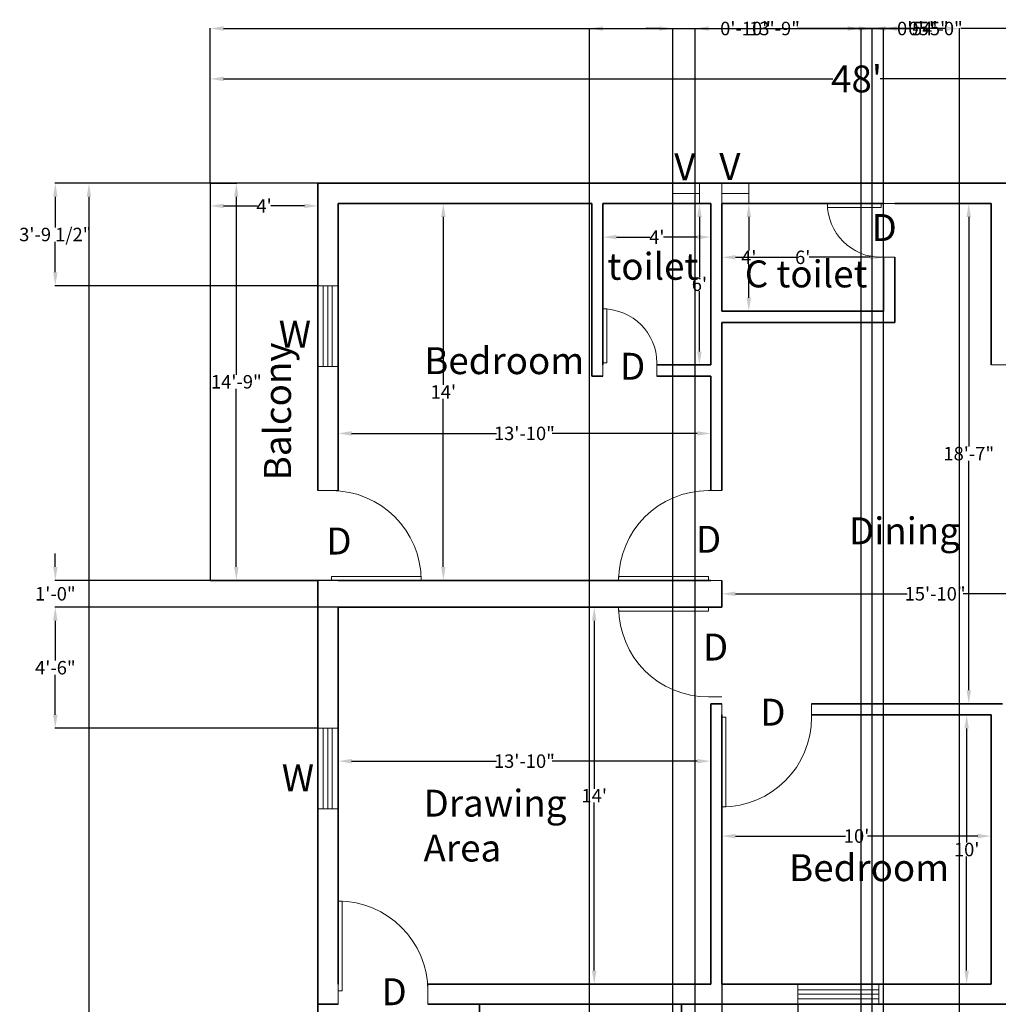
# Model space of a CAD drawing. Units: inches. Extents: x 1936 to 2761, y 1431 to 2889.
# Tile 5 of 6: x 1936 to 2372, y 2451 to 2889. Entities that reach past the tile are written whole.
import ezdxf

# ---------------------------------------------------------------- set-up
doc = ezdxf.new("R2010")
doc.units = ezdxf.units.IN
doc.header["$MEASUREMENT"] = 0
for name, color, linetype, lineweight in [('A-ANNO-DIMS', 172, 'Continuous', 13), ('A-ANNO-TEXT', 50, 'Continuous', 18), ('A-AREA-IDEN', 50, 'Continuous', 18), ('A-FLOR-EDGE', 4, 'Continuous', 25), ('A-FLOR-EVTR', 4, 'Continuous', 35), ('A-FLOR-FIXT', 8, 'Continuous', 18), ('A-GLAZ', 3, 'Continuous', 18), ('A-WALL', 4, 'Continuous', 35), ('doors', 10, 'Continuous', 18)]:
    doc.layers.add(name, color=color, linetype=linetype, lineweight=lineweight)
doc.styles.get("Standard").update_dxf_attribs({"font": 'arial.ttf'})
doc.dimstyles.get("Standard").update_dxf_attribs({"dimtxt": 6, "dimasz": 6, "dimexe": 0.18, "dimexo": 0.0625, "dimgap": 0.09, "dimtad": 0, "dimtih": 1, "dimtoh": 1, "dimdec": 0, "dimzin": 0, "dimdsep": 46, "dimlunit": 3, "dimtxsty": 'Standard', "dimcen": 0.09, "dimadec": 0, "dimazin": 0, "dimtfac": 1, "dimtdec": 0, "dimtofl": 0, "dimtmove": 0, "dimatfit": 3, "dimfxl": 1, "dimtolj": 1, "dimtzin": 0, "dimarcsym": 0})

# ---------------------------------------------------------------- blocks, each defined once
blk = doc.blocks.new('*U4')
for p, q in [((0, 0), (0, 6)), ((24, 0), (24, 6))]:
    blk.add_line(p, q)
blk.add_lwpolyline([(0, 0), (0, -24), (1.75, -24), (1.75, 0)], close=True)
blk.add_arc((0, 0), 24, 270, 0)
blk = doc.blocks.new('*U3')
for p, q in [((0, 0), (0, -6)), ((24, 0), (24, -6))]:
    blk.add_line(p, q)
blk.add_lwpolyline([(0, 0), (0, 24), (1.75, 24), (1.75, 0)], close=True)
blk.add_arc((0, 0), 24, 0, 90)
blk = doc.blocks.new('*U5')
for p, q in [((0, 0), (0, -6)), ((40, 0), (40, -6))]:
    blk.add_line(p, q)
blk.add_lwpolyline([(0, 0), (0, 40), (1.75, 40), (1.75, 0)], close=True)
blk.add_arc((0, 0), 40, 0, 90)
blk = doc.blocks.new('*U2')
for p, q in [((0, 0), (0, 6)), ((40, 0), (40, 6))]:
    blk.add_line(p, q)
blk.add_lwpolyline([(0, 0), (0, -40), (1.75, -40), (1.75, 0)], close=True)
blk.add_arc((0, 0), 40, 270, 360)
blk = doc.blocks.new('*U6')
for p, q in [((0, 0), (0, -6)), ((40, 0), (40, -6))]:
    blk.add_line(p, q)
blk.add_lwpolyline([(0, 0), (0, 40), (1.75, 40), (1.75, 0)], close=True)
blk.add_arc((0, 0), 40, 0, 90)
blk = doc.blocks.new('*U7')
for p, q in [((0, 0), (0, 6)), ((40, 0), (40, 6))]:
    blk.add_line(p, q)
blk.add_lwpolyline([(0, 0), (0, -40), (1.75, -40), (1.75, 0)], close=True)
blk.add_arc((0, 0), 40, 270, 0)
blk = doc.blocks.new('*D8')
at = {"layer": 'A-ANNO-DIMS', "color": 0, "lineweight": -2, "transparency": 16777216}
for p, q in [((2078.01, 2697.85), (2078.01, 2705.23)), ((2084.01, 2705.05), (2148.56, 2705.05)), ((2238.01, 2705.05), (2173.45, 2705.05)), ((2244.01, 2697.85), (2244.01, 2705.23))]:
    blk.add_line(p, q, dxfattribs=at)
at = {"layer": 'A-ANNO-DIMS', "color": 0, "transparency": 16777216}
for points in [[(2084.01, 2706.05), (2084.01, 2704.05), (2078.01, 2705.05)], [(2238.01, 2706.05), (2238.01, 2704.05), (2244.01, 2705.05)]]:
    blk.add_solid(points, dxfattribs=at)
at = {"layer": 'Defpoints', "color": 0, "transparency": 16777216}
for p in [(2244.01, 2705.05), (2078.01, 2697.79), (2244.01, 2697.79)]:
    blk.add_point(p, dxfattribs=at)
at = {"layer": 'A-ANNO-DIMS', "color": 0, "transparency": 16777216, "insert": (2161.01, 2705.05), "char_height": 6, "attachment_point": 5}
blk.add_mtext('\\A1;13\'-10"', dxfattribs=at)
blk = doc.blocks.new('*D9')
at = {"layer": 'A-ANNO-DIMS', "color": 0, "lineweight": -2, "transparency": 16777216}
for p, q in [((2124.95, 2807.55), (2125.07, 2807.55)), ((2124.89, 2801.55), (2124.89, 2726.65)), ((2124.89, 2645.55), (2124.89, 2720.45)), ((2124.95, 2639.55), (2125.07, 2639.55))]:
    blk.add_line(p, q, dxfattribs=at)
at = {"layer": 'A-ANNO-DIMS', "color": 0, "transparency": 16777216}
for points in [[(2123.89, 2801.55), (2125.89, 2801.55), (2124.89, 2807.55)], [(2123.89, 2645.55), (2125.89, 2645.55), (2124.89, 2639.55)]]:
    blk.add_solid(points, dxfattribs=at)
at = {"layer": 'Defpoints', "color": 0, "transparency": 16777216}
for p in [(2124.89, 2807.55), (2124.89, 2639.55), (2124.89, 2639.55)]:
    blk.add_point(p, dxfattribs=at)
at = {"layer": 'A-ANNO-DIMS', "color": 0, "transparency": 16777216, "insert": (2124.89, 2723.55), "char_height": 6, "attachment_point": 5}
blk.add_mtext("\\A1;14'", dxfattribs=at)
blk = doc.blocks.new('*D10')
at = {"layer": 'A-ANNO-DIMS', "color": 0, "lineweight": -2, "transparency": 16777216}
for p, q in [((2249.01, 2633.61), (2249.01, 2633.73)), ((2439.01, 2633.61), (2439.01, 2633.73)), ((2255.01, 2633.55), (2331.56, 2633.55)), ((2433.01, 2633.55), (2356.45, 2633.55))]:
    blk.add_line(p, q, dxfattribs=at)
at = {"layer": 'A-ANNO-DIMS', "color": 0, "transparency": 16777216}
for points in [[(2255.01, 2634.55), (2255.01, 2632.55), (2249.01, 2633.55)], [(2433.01, 2634.55), (2433.01, 2632.55), (2439.01, 2633.55)]]:
    blk.add_solid(points, dxfattribs=at)
at = {"layer": 'Defpoints', "color": 0, "transparency": 16777216}
for p in [(2249.01, 2633.55), (2439.01, 2633.55), (2439.01, 2633.55)]:
    blk.add_point(p, dxfattribs=at)
at = {"layer": 'A-ANNO-DIMS', "color": 0, "transparency": 16777216, "insert": (2344.01, 2633.55), "char_height": 6, "attachment_point": 5}
blk.add_mtext('\\A1;15\'-10"', dxfattribs=at)
blk = doc.blocks.new('*D11')
at = {"layer": 'A-ANNO-DIMS', "color": 0, "lineweight": -2, "transparency": 16777216}
for p, q in [((2347.57, 2807.55), (2359.19, 2807.55)), ((2359.01, 2801.55), (2359.01, 2699.2)), ((2359.01, 2590.55), (2359.01, 2692.9)), ((2347.57, 2584.55), (2359.19, 2584.55))]:
    blk.add_line(p, q, dxfattribs=at)
at = {"layer": 'A-ANNO-DIMS', "color": 0, "transparency": 16777216}
for points in [[(2358.01, 2801.55), (2360.01, 2801.55), (2359.01, 2807.55)], [(2358.01, 2590.55), (2360.01, 2590.55), (2359.01, 2584.55)]]:
    blk.add_solid(points, dxfattribs=at)
at = {"layer": 'Defpoints', "color": 0, "transparency": 16777216}
for p in [(2347.51, 2807.55), (2347.51, 2584.55), (2359.01, 2584.55)]:
    blk.add_point(p, dxfattribs=at)
at = {"layer": 'A-ANNO-DIMS', "color": 0, "transparency": 16777216, "insert": (2359.01, 2696.05), "char_height": 6, "attachment_point": 5}
blk.add_mtext('\\A1;18\'-7"', dxfattribs=at)
blk = doc.blocks.new('*D16')
at = {"layer": 'A-ANNO-DIMS', "color": 0, "lineweight": -2, "transparency": 16777216}
for p, q in [((2249.01, 2783.61), (2249.01, 2783.73)), ((2255.01, 2783.55), (2282.14, 2783.55)), ((2315.01, 2783.55), (2287.87, 2783.55)), ((2321.01, 2783.49), (2321.01, 2783.37))]:
    blk.add_line(p, q, dxfattribs=at)
at = {"layer": 'A-ANNO-DIMS', "color": 0, "transparency": 16777216}
for points in [[(2255.01, 2784.55), (2255.01, 2782.55), (2249.01, 2783.55)], [(2315.01, 2784.55), (2315.01, 2782.55), (2321.01, 2783.55)]]:
    blk.add_solid(points, dxfattribs=at)
at = {"layer": 'Defpoints', "color": 0, "transparency": 16777216}
for p in [(2249.01, 2783.55), (2321.01, 2783.55), (2321.01, 2783.55)]:
    blk.add_point(p, dxfattribs=at)
at = {"layer": 'A-ANNO-DIMS', "color": 0, "transparency": 16777216, "insert": (2285.01, 2783.55), "char_height": 6, "attachment_point": 5}
blk.add_mtext("\\A1;6'", dxfattribs=at)
blk = doc.blocks.new('*D17')
at = {"layer": 'A-ANNO-DIMS', "color": 0, "lineweight": -2, "transparency": 16777216}
for p, q in [((2261.07, 2807.55), (2261.19, 2807.55)), ((2261.01, 2801.55), (2261.01, 2786.64)), ((2261.01, 2765.55), (2261.01, 2780.46)), ((2261.07, 2759.55), (2261.19, 2759.55))]:
    blk.add_line(p, q, dxfattribs=at)
at = {"layer": 'A-ANNO-DIMS', "color": 0, "transparency": 16777216}
for points in [[(2260.01, 2801.55), (2262.01, 2801.55), (2261.01, 2807.55)], [(2260.01, 2765.55), (2262.01, 2765.55), (2261.01, 2759.55)]]:
    blk.add_solid(points, dxfattribs=at)
at = {"layer": 'Defpoints', "color": 0, "transparency": 16777216}
for p in [(2261.01, 2807.55), (2261.01, 2759.55), (2261.01, 2759.55)]:
    blk.add_point(p, dxfattribs=at)
at = {"layer": 'A-ANNO-DIMS', "color": 0, "transparency": 16777216, "insert": (2261.01, 2783.55), "char_height": 6, "attachment_point": 5}
blk.add_mtext("\\A1;4'", dxfattribs=at)
blk = doc.blocks.new('*D18')
at = {"layer": 'A-ANNO-DIMS', "color": 0, "lineweight": -2, "transparency": 16777216}
for p, q in [((2234.79, 2807.55), (2239.17, 2807.55)), ((2238.99, 2801.55), (2238.99, 2774.7)), ((2238.99, 2741.55), (2238.99, 2768.4)), ((2234.79, 2735.55), (2239.17, 2735.55))]:
    blk.add_line(p, q, dxfattribs=at)
at = {"layer": 'A-ANNO-DIMS', "color": 0, "transparency": 16777216}
for points in [[(2237.99, 2801.55), (2239.99, 2801.55), (2238.99, 2807.55)], [(2237.99, 2741.55), (2239.99, 2741.55), (2238.99, 2735.55)]]:
    blk.add_solid(points, dxfattribs=at)
at = {"layer": 'Defpoints', "color": 0, "transparency": 16777216}
for p in [(2234.73, 2807.55), (2234.73, 2735.55), (2238.99, 2735.55)]:
    blk.add_point(p, dxfattribs=at)
at = {"layer": 'A-ANNO-DIMS', "color": 0, "transparency": 16777216, "insert": (2238.99, 2771.55), "char_height": 6, "attachment_point": 5}
blk.add_mtext("\\A1;6'", dxfattribs=at)
blk = doc.blocks.new('*D19')
at = {"layer": 'A-ANNO-DIMS', "color": 0, "lineweight": -2, "transparency": 16777216}
for p, q in [((2196.01, 2792.63), (2196.01, 2792.74)), ((2202.01, 2792.56), (2217.03, 2792.56)), ((2238.01, 2792.56), (2222.98, 2792.56)), ((2244.01, 2792.63), (2244.01, 2792.74))]:
    blk.add_line(p, q, dxfattribs=at)
at = {"layer": 'A-ANNO-DIMS', "color": 0, "transparency": 16777216}
for points in [[(2202.01, 2793.56), (2202.01, 2791.56), (2196.01, 2792.56)], [(2238.01, 2793.56), (2238.01, 2791.56), (2244.01, 2792.56)]]:
    blk.add_solid(points, dxfattribs=at)
at = {"layer": 'Defpoints', "color": 0, "transparency": 16777216}
for p in [(2196.01, 2792.56), (2196.01, 2792.56), (2244.01, 2792.56)]:
    blk.add_point(p, dxfattribs=at)
at = {"layer": 'A-ANNO-DIMS', "color": 0, "transparency": 16777216, "insert": (2220.01, 2792.56), "char_height": 6, "attachment_point": 5}
blk.add_mtext("\\A1;4'", dxfattribs=at)
blk = doc.blocks.new('*D20')
at = {"layer": 'A-ANNO-DIMS', "color": 0, "lineweight": -2, "transparency": 16777216}
for p, q in [((2078.01, 2559.01), (2078.01, 2559.13)), ((2244.01, 2559.01), (2244.01, 2559.13)), ((2084.01, 2558.95), (2148.56, 2558.95)), ((2238.01, 2558.95), (2173.45, 2558.95))]:
    blk.add_line(p, q, dxfattribs=at)
at = {"layer": 'A-ANNO-DIMS', "color": 0, "transparency": 16777216}
for points in [[(2084.01, 2559.95), (2084.01, 2557.95), (2078.01, 2558.95)], [(2238.01, 2559.95), (2238.01, 2557.95), (2244.01, 2558.95)]]:
    blk.add_solid(points, dxfattribs=at)
at = {"layer": 'Defpoints', "color": 0, "transparency": 16777216}
for p in [(2078.01, 2558.95), (2244.01, 2558.95), (2244.01, 2558.95)]:
    blk.add_point(p, dxfattribs=at)
at = {"layer": 'A-ANNO-DIMS', "color": 0, "transparency": 16777216, "insert": (2161.01, 2558.95), "char_height": 6, "attachment_point": 5}
blk.add_mtext('\\A1;13\'-10"', dxfattribs=at)
blk = doc.blocks.new('*D21')
at = {"layer": 'A-ANNO-DIMS', "color": 0, "lineweight": -2, "transparency": 16777216}
for p, q in [((2187.65, 2627.55), (2192.3, 2627.55)), ((2192.12, 2621.55), (2192.12, 2546.65)), ((2192.12, 2465.55), (2192.12, 2540.45)), ((2187.65, 2459.55), (2192.3, 2459.55))]:
    blk.add_line(p, q, dxfattribs=at)
at = {"layer": 'A-ANNO-DIMS', "color": 0, "transparency": 16777216}
for points in [[(2191.12, 2621.55), (2193.12, 2621.55), (2192.12, 2627.55)], [(2191.12, 2465.55), (2193.12, 2465.55), (2192.12, 2459.55)]]:
    blk.add_solid(points, dxfattribs=at)
at = {"layer": 'Defpoints', "color": 0, "transparency": 16777216}
for p in [(2187.59, 2627.55), (2187.59, 2459.55), (2192.12, 2459.55)]:
    blk.add_point(p, dxfattribs=at)
at = {"layer": 'A-ANNO-DIMS', "color": 0, "transparency": 16777216, "insert": (2192.12, 2543.55), "char_height": 6, "attachment_point": 5}
blk.add_mtext("\\A1;14'", dxfattribs=at)
blk = doc.blocks.new('*D22')
at = {"layer": 'A-ANNO-DIMS', "color": 0, "lineweight": -2, "transparency": 16777216}
for p, q in [((2249.01, 2519.61), (2249.01, 2525.73)), ((2255.01, 2525.55), (2304.11, 2525.55)), ((2363.01, 2525.55), (2313.91, 2525.55)), ((2369.01, 2519.61), (2369.01, 2525.73))]:
    blk.add_line(p, q, dxfattribs=at)
at = {"layer": 'A-ANNO-DIMS', "color": 0, "transparency": 16777216}
for points in [[(2255.01, 2526.55), (2255.01, 2524.55), (2249.01, 2525.55)], [(2363.01, 2526.55), (2363.01, 2524.55), (2369.01, 2525.55)]]:
    blk.add_solid(points, dxfattribs=at)
at = {"layer": 'Defpoints', "color": 0, "transparency": 16777216}
for p in [(2249.01, 2525.55), (2249.01, 2519.55), (2369.01, 2519.55)]:
    blk.add_point(p, dxfattribs=at)
at = {"layer": 'A-ANNO-DIMS', "color": 0, "transparency": 16777216, "insert": (2309.01, 2525.55), "char_height": 6, "attachment_point": 5}
blk.add_mtext("\\A1;10'", dxfattribs=at)
blk = doc.blocks.new('*D23')
at = {"layer": 'A-ANNO-DIMS', "color": 0, "lineweight": -2, "transparency": 16777216}
for p, q in [((2354.08, 2579.55), (2358.25, 2579.55)), ((2358.07, 2573.55), (2358.07, 2522.7)), ((2358.07, 2465.55), (2358.07, 2516.4)), ((2354.08, 2459.55), (2358.25, 2459.55))]:
    blk.add_line(p, q, dxfattribs=at)
at = {"layer": 'A-ANNO-DIMS', "color": 0, "transparency": 16777216}
for points in [[(2357.07, 2573.55), (2359.07, 2573.55), (2358.07, 2579.55)], [(2357.07, 2465.55), (2359.07, 2465.55), (2358.07, 2459.55)]]:
    blk.add_solid(points, dxfattribs=at)
at = {"layer": 'Defpoints', "color": 0, "transparency": 16777216}
for p in [(2354.02, 2579.55), (2354.02, 2459.55), (2358.07, 2459.55)]:
    blk.add_point(p, dxfattribs=at)
at = {"layer": 'A-ANNO-DIMS', "color": 0, "transparency": 16777216, "insert": (2358.07, 2519.55), "char_height": 6, "attachment_point": 5}
blk.add_mtext("\\A1;10'", dxfattribs=at)
blk = doc.blocks.new('*D26')
at = {"layer": 'A-ANNO-DIMS', "color": 0, "lineweight": -2, "transparency": 16777216}
for p, q in [((2021.01, 2816.49), (2021.01, 2806.29)), ((2069.01, 2816.49), (2069.01, 2806.29)), ((2027.01, 2806.47), (2042.03, 2806.47)), ((2063.01, 2806.47), (2047.98, 2806.47))]:
    blk.add_line(p, q, dxfattribs=at)
at = {"layer": 'A-ANNO-DIMS', "color": 0, "transparency": 16777216}
for points in [[(2027.01, 2807.47), (2027.01, 2805.47), (2021.01, 2806.47)], [(2063.01, 2807.47), (2063.01, 2805.47), (2069.01, 2806.47)]]:
    blk.add_solid(points, dxfattribs=at)
at = {"layer": 'Defpoints', "color": 0, "transparency": 16777216}
for p in [(2021.01, 2816.55), (2069.01, 2816.55), (2021.01, 2806.47)]:
    blk.add_point(p, dxfattribs=at)
at = {"layer": 'A-ANNO-DIMS', "color": 0, "transparency": 16777216, "insert": (2045.01, 2806.47), "char_height": 6, "attachment_point": 5}
blk.add_mtext("\\A1;4'", dxfattribs=at)
blk = doc.blocks.new('*D27')
at = {"layer": 'A-ANNO-DIMS', "color": 0, "lineweight": -2, "transparency": 16777216}
for p, q in [((2021.07, 2816.55), (2032.84, 2816.55)), ((2032.66, 2810.55), (2032.66, 2731.2)), ((2032.66, 2645.55), (2032.66, 2724.9)), ((2021.07, 2639.55), (2032.84, 2639.55))]:
    blk.add_line(p, q, dxfattribs=at)
at = {"layer": 'A-ANNO-DIMS', "color": 0, "transparency": 16777216}
for points in [[(2031.66, 2810.55), (2033.66, 2810.55), (2032.66, 2816.55)], [(2031.66, 2645.55), (2033.66, 2645.55), (2032.66, 2639.55)]]:
    blk.add_solid(points, dxfattribs=at)
at = {"layer": 'Defpoints', "color": 0, "transparency": 16777216}
for p in [(2021.01, 2816.55), (2021.01, 2639.55), (2032.66, 2639.55)]:
    blk.add_point(p, dxfattribs=at)
at = {"layer": 'A-ANNO-DIMS', "color": 0, "transparency": 16777216, "insert": (2032.66, 2728.05), "char_height": 6, "attachment_point": 5}
blk.add_mtext('\\A1;14\'-9"', dxfattribs=at)
blk = doc.blocks.new('*D76')
at = {"layer": 'A-ANNO-DIMS', "color": 0, "lineweight": -2, "transparency": 16777216}
for p, q in [((2068.94, 2816.55), (1966.82, 2816.55)), ((1967, 2810.55), (1967, 2168.77)), ((1967, 1514.55), (1967, 2156.33)), ((2068.94, 1508.55), (1966.82, 1508.55))]:
    blk.add_line(p, q, dxfattribs=at)
at = {"layer": 'A-ANNO-DIMS', "color": 0, "transparency": 16777216}
for points in [[(1966, 2810.55), (1968, 2810.55), (1967, 2816.55)], [(1966, 1514.55), (1968, 1514.55), (1967, 1508.55)]]:
    blk.add_solid(points, dxfattribs=at)
at = {"layer": 'Defpoints', "color": 0, "transparency": 16777216}
for p in [(2069.01, 2816.55), (1967, 1508.55), (2069.01, 1508.55)]:
    blk.add_point(p, dxfattribs=at)
at = {"layer": 'A-ANNO-DIMS', "color": 0, "transparency": 16777216, "insert": (1967, 2162.55), "char_height": 6, "attachment_point": 5}
blk.add_mtext("\\A1;{\\H2x;109'}", dxfattribs=at)
blk = doc.blocks.new('*D80')
at = {"layer": 'A-ANNO-DIMS', "color": 0, "lineweight": -2, "transparency": 16777216}
for p, q in [((2021.01, 2816.61), (2021.01, 2863.26)), ((2027.01, 2863.08), (2298.49, 2863.08)), ((2591.01, 2863.08), (2319.52, 2863.08)), ((2597.01, 2816.61), (2597.01, 2863.26))]:
    blk.add_line(p, q, dxfattribs=at)
at = {"layer": 'A-ANNO-DIMS', "color": 0, "transparency": 16777216}
for points in [[(2027.01, 2864.08), (2027.01, 2862.08), (2021.01, 2863.08)], [(2591.01, 2864.08), (2591.01, 2862.08), (2597.01, 2863.08)]]:
    blk.add_solid(points, dxfattribs=at)
at = {"layer": 'Defpoints', "color": 0, "transparency": 16777216}
for p in [(2021.01, 2863.08), (2021.01, 2816.55), (2597.01, 2816.55)]:
    blk.add_point(p, dxfattribs=at)
at = {"layer": 'A-ANNO-DIMS', "color": 0, "transparency": 16777216, "insert": (2309.01, 2863.08), "char_height": 6, "attachment_point": 5}
blk.add_mtext("\\A1;{\\H2x;48'}", dxfattribs=at)
blk = doc.blocks.new('WIN-36')
for p, q in [((0, 9), (0, 0)), ((36, 9), (36, 0)), ((36, 6.5), (0, 6.5)), ((36, 4.5), (0, 4.5)), ((36, 2.5), (0, 2.5))]:
    blk.add_line(p, q)
blk = doc.blocks.new('VENT-12')
for p, q in [((0, 0), (0, 9)), ((12, 0), (12, 9)), ((0, 4.5), (12, 4.5))]:
    blk.add_line(p, q)
blk = doc.blocks.new('COUNTER-KITCHEN-U')
for p, q in [((41, 36), (41, 0)), ((41, 36), (135, 36)), ((135, 36), (135, 0)), ((0, 0), (41, 0)), ((135, 0), (171, 0))]:
    blk.add_line(p, q)
blk = doc.blocks.new('*D99')
at = {"layer": 'A-ANNO-DIMS', "color": 0, "lineweight": -2, "transparency": 16777216}
for p, q in [((2021.01, 2816.61), (2021.01, 2885.73)), ((2027.01, 2885.55), (2334.61, 2885.55)), ((2663.01, 2885.55), (2355.4, 2885.55)), ((2669.01, 2360.61), (2669.01, 2885.73))]:
    blk.add_line(p, q, dxfattribs=at)
at = {"layer": 'A-ANNO-DIMS', "color": 0, "transparency": 16777216}
for points in [[(2027.01, 2886.55), (2027.01, 2884.55), (2021.01, 2885.55)], [(2663.01, 2886.55), (2663.01, 2884.55), (2669.01, 2885.55)]]:
    blk.add_solid(points, dxfattribs=at)
at = {"layer": 'Defpoints', "color": 0, "transparency": 16777216}
for p in [(2669.01, 2885.55), (2021.01, 2816.55), (2669.01, 2360.55)]:
    blk.add_point(p, dxfattribs=at)
at = {"layer": 'A-ANNO-DIMS', "color": 0, "transparency": 16777216, "insert": (2345.01, 2885.55), "char_height": 6, "attachment_point": 5}
blk.add_mtext('\\A1;54\'-0"', dxfattribs=at)
blk = doc.blocks.new('*D104')
at = {"layer": 'A-ANNO-DIMS', "color": 0, "lineweight": -2, "transparency": 16777216}
for p, q in [((2190.01, 1922.61), (2190.01, 2885.73)), ((2196.01, 2885.55), (2262.35, 2885.55)), ((2348.92, 2885.55), (2282.58, 2885.55)), ((2354.92, 1922.61), (2354.92, 2885.73))]:
    blk.add_line(p, q, dxfattribs=at)
at = {"layer": 'A-ANNO-DIMS', "color": 0, "transparency": 16777216}
for points in [[(2196.01, 2886.55), (2196.01, 2884.55), (2190.01, 2885.55)], [(2348.92, 2886.55), (2348.92, 2884.55), (2354.92, 2885.55)]]:
    blk.add_solid(points, dxfattribs=at)
at = {"layer": 'Defpoints', "color": 0, "transparency": 16777216}
for p in [(2354.92, 2885.55), (2190.01, 1922.55), (2354.92, 1922.55)]:
    blk.add_point(p, dxfattribs=at)
at = {"layer": 'A-ANNO-DIMS', "color": 0, "transparency": 16777216, "insert": (2272.46, 2885.55), "char_height": 6, "attachment_point": 5}
blk.add_mtext('\\A1;13\'-9"', dxfattribs=at)
blk = doc.blocks.new('*D107')
at = {"layer": 'A-ANNO-DIMS', "color": 0, "lineweight": -2, "transparency": 16777216}
for p, q in [((2221.14, 2885.55), (2215.14, 2885.55)), ((2227.14, 1922.61), (2227.14, 2885.73)), ((2237.14, 1922.61), (2237.14, 2885.73)), ((2243.14, 2885.55), (2249.14, 2885.55))]:
    blk.add_line(p, q, dxfattribs=at)
at = {"layer": 'A-ANNO-DIMS', "color": 0, "transparency": 16777216}
for points in [[(2221.14, 2886.55), (2221.14, 2884.55), (2227.14, 2885.55)], [(2243.14, 2886.55), (2243.14, 2884.55), (2237.14, 2885.55)]]:
    blk.add_solid(points, dxfattribs=at)
at = {"layer": 'Defpoints', "color": 0, "transparency": 16777216}
for p in [(2237.14, 2885.55), (2227.14, 1922.55), (2237.14, 1922.55)]:
    blk.add_point(p, dxfattribs=at)
at = {"layer": 'A-ANNO-DIMS', "color": 0, "transparency": 16777216, "insert": (2259.54, 2885.55), "char_height": 6, "attachment_point": 5}
blk.add_mtext('\\A1;0\'-10"', dxfattribs=at)
blk = doc.blocks.new('*D111')
at = {"layer": 'A-ANNO-DIMS', "color": 0, "lineweight": -2, "transparency": 16777216}
for p, q in [((2310.01, 2885.55), (2304.01, 2885.55)), ((2316.01, 2351.61), (2316.01, 2885.73)), ((2321.01, 2351.61), (2321.01, 2885.73)), ((2327.01, 2885.55), (2333.01, 2885.55))]:
    blk.add_line(p, q, dxfattribs=at)
at = {"layer": 'A-ANNO-DIMS', "color": 0, "transparency": 16777216}
for points in [[(2310.01, 2886.55), (2310.01, 2884.55), (2316.01, 2885.55)], [(2327.01, 2886.55), (2327.01, 2884.55), (2321.01, 2885.55)]]:
    blk.add_solid(points, dxfattribs=at)
at = {"layer": 'Defpoints', "color": 0, "transparency": 16777216}
for p in [(2321.01, 2885.55), (2316.01, 2351.55), (2321.01, 2351.55)]:
    blk.add_point(p, dxfattribs=at)
at = {"layer": 'A-ANNO-DIMS', "color": 0, "transparency": 16777216, "insert": (2341.07, 2885.55), "char_height": 6, "attachment_point": 5}
blk.add_mtext('\\A1;0\'-5"', dxfattribs=at)
blk = doc.blocks.new('*D114')
at = {"layer": 'A-ANNO-DIMS', "color": 0, "lineweight": -2, "transparency": 16777216}
for p, q in [((2305.01, 2885.55), (2299.01, 2885.55)), ((2311.01, 2351.61), (2311.01, 2885.73)), ((2316.01, 2351.61), (2316.01, 2885.73)), ((2322.01, 2885.55), (2328.01, 2885.55))]:
    blk.add_line(p, q, dxfattribs=at)
at = {"layer": 'A-ANNO-DIMS', "color": 0, "transparency": 16777216}
for points in [[(2305.01, 2886.55), (2305.01, 2884.55), (2311.01, 2885.55)], [(2322.01, 2886.55), (2322.01, 2884.55), (2316.01, 2885.55)]]:
    blk.add_solid(points, dxfattribs=at)
at = {"layer": 'Defpoints', "color": 0, "transparency": 16777216}
for p in [(2316.01, 2885.55), (2311.01, 2351.55), (2316.01, 2351.55)]:
    blk.add_point(p, dxfattribs=at)
at = {"layer": 'A-ANNO-DIMS', "color": 0, "transparency": 16777216, "insert": (2336.07, 2885.55), "char_height": 6, "attachment_point": 5}
blk.add_mtext('\\A1;0\'-5"', dxfattribs=at)
blk = doc.blocks.new('*D118')
at = {"layer": 'A-ANNO-DIMS', "color": 0, "lineweight": -2, "transparency": 16777216}
for p, q in [((2068.94, 2816.55), (1951.83, 2816.55)), ((1952.01, 2810.55), (1952.01, 2796.91)), ((1952.01, 2776.89), (1952.01, 2790.53)), ((2068.84, 2770.89), (1951.83, 2770.89))]:
    blk.add_line(p, q, dxfattribs=at)
at = {"layer": 'A-ANNO-DIMS', "color": 0, "transparency": 16777216}
for points in [[(1951.01, 2810.55), (1953.01, 2810.55), (1952.01, 2816.55)], [(1951.01, 2776.89), (1953.01, 2776.89), (1952.01, 2770.89)]]:
    blk.add_solid(points, dxfattribs=at)
at = {"layer": 'Defpoints', "color": 0, "transparency": 16777216}
for p in [(2069.01, 2816.55), (1952.01, 2770.89), (2068.9, 2770.89)]:
    blk.add_point(p, dxfattribs=at)
at = {"layer": 'A-ANNO-DIMS', "color": 0, "transparency": 16777216, "insert": (1952.01, 2793.72), "char_height": 6, "attachment_point": 5}
blk.add_mtext('\\A1;3\'-9 1/2"', dxfattribs=at)
blk = doc.blocks.new('*D119')
at = {"layer": 'A-ANNO-DIMS', "color": 0, "lineweight": -2, "transparency": 16777216}
for p, q in [((2077.94, 2627.55), (1951.83, 2627.55)), ((1952.01, 2621.55), (1952.01, 2603.76)), ((1952.01, 2579.66), (1952.01, 2597.45)), ((2068.84, 2573.66), (1951.83, 2573.66))]:
    blk.add_line(p, q, dxfattribs=at)
at = {"layer": 'A-ANNO-DIMS', "color": 0, "transparency": 16777216}
for points in [[(1951.01, 2621.55), (1953.01, 2621.55), (1952.01, 2627.55)], [(1951.01, 2579.66), (1953.01, 2579.66), (1952.01, 2573.66)]]:
    blk.add_solid(points, dxfattribs=at)
at = {"layer": 'Defpoints', "color": 0, "transparency": 16777216}
for p in [(2078.01, 2627.55), (1952.01, 2573.66), (2068.9, 2573.66)]:
    blk.add_point(p, dxfattribs=at)
at = {"layer": 'A-ANNO-DIMS', "color": 0, "transparency": 16777216, "insert": (1952.01, 2600.6), "char_height": 6, "attachment_point": 5}
blk.add_mtext('\\A1;4\'-6"', dxfattribs=at)
blk = doc.blocks.new('*D120')
at = {"layer": 'A-ANNO-DIMS', "color": 0, "lineweight": -2, "transparency": 16777216}
for p, q in [((2249.01, 2459.49), (2249.01, 1439.37)), ((2282.92, 2450.49), (2282.92, 1439.37)), ((2255.01, 1439.55), (2255.52, 1439.55)), ((2276.92, 1439.55), (2276.41, 1439.55))]:
    blk.add_line(p, q, dxfattribs=at)
at = {"layer": 'A-ANNO-DIMS', "color": 0, "transparency": 16777216}
for points in [[(2255.01, 1440.55), (2255.01, 1438.55), (2249.01, 1439.55)], [(2276.92, 1440.55), (2276.92, 1438.55), (2282.92, 1439.55)]]:
    blk.add_solid(points, dxfattribs=at)
at = {"layer": 'Defpoints', "color": 0, "transparency": 16777216}
for p in [(2249.01, 2459.55), (2282.92, 2450.55), (2282.92, 1439.55)]:
    blk.add_point(p, dxfattribs=at)
at = {"layer": 'A-ANNO-DIMS', "color": 0, "transparency": 16777216, "insert": (2265.96, 1439.55), "char_height": 6, "attachment_point": 5}
blk.add_mtext('\\A1;2\'-10"', dxfattribs=at)
blk = doc.blocks.new('*D122')
at = {"layer": 'A-ANNO-DIMS', "color": 0, "lineweight": -2, "transparency": 16777216}
for p, q in [((1952.006183, 2645.549411), (1952.006183, 2651.549411)), ((2077.943683, 2639.549411), (1951.826183, 2639.549411)), ((2077.943683, 2627.549411), (1951.826183, 2627.549411)), ((1952.006183, 2621.549411), (1952.006183, 2615.549411))]:
    blk.add_line(p, q, dxfattribs=at)
at = {"layer": 'A-ANNO-DIMS', "color": 0, "transparency": 16777216}
for points in [[(1951.006183, 2645.549411), (1953.006183, 2645.549411), (1952.006183, 2639.549411)], [(1951.006183, 2621.549411), (1953.006183, 2621.549411), (1952.006183, 2627.549411)]]:
    blk.add_solid(points, dxfattribs=at)
at = {"layer": 'Defpoints', "color": 0, "transparency": 16777216}
for p in [(2078.006183, 2639.549411), (1952.006183, 2627.549411), (2078.006183, 2627.549411)]:
    blk.add_point(p, dxfattribs=at)
at = {"layer": 'A-ANNO-DIMS', "color": 0, "transparency": 16777216, "insert": (1952.006183, 2633.549411), "char_height": 6, "attachment_point": 5}
blk.add_mtext('\\A1;1\'-0"', dxfattribs=at)

msp = doc.modelspace()

# ---------------------------------------------------------------- linework, layer by layer
at = {"layer": 'A-FLOR-EDGE'}
for p, q in [((2069.01, 2816.55), (2021.01, 2816.55)), ((2021.01, 2816.55), (2021.01, 2639.55)), ((2021.01, 2639.55), (2069.01, 2639.55))]:
    msp.add_line(p, q, dxfattribs=at)
at = {"layer": 'A-FLOR-EVTR'}
for p, q in [((2141.01, 2450.55), (2231.01, 2450.55)), ((2141.01, 2441.55), (2141.01, 2450.55)), ((2231.01, 2450.55), (2231.01, 2360.55))]:
    msp.add_line(p, q, dxfattribs=at)
at = {"layer": 'A-WALL'}
for p, q in [((2069.01, 2816.55), (2549.01, 2816.55)), ((2069.01, 2679.55), (2069.01, 2816.55)), ((2078.01, 2679.55), (2078.01, 2807.55)), ((2078.01, 2807.55), (2191.01, 2807.55)), ((2191.01, 2730.55), (2191.01, 2807.55)), ((2196.01, 2735.55), (2196.01, 2807.55)), ((2196.01, 2807.55), (2244.01, 2807.55)), ((2244.01, 2735.55), (2244.01, 2807.55)), ((2249.01, 2807.55), (2321.01, 2807.55)), ((2249.01, 2759.55), (2249.01, 2807.55)), ((2326.01, 2807.55), (2369.01, 2807.55)), ((2369.01, 2807.55), (2369.01, 2735.55)), ((2321.01, 2759.55), (2321.01, 2783.55)), ((2326.01, 2754.55), (2326.01, 2783.55)), ((2249.01, 2759.55), (2321.01, 2759.55)), ((2249.01, 2754.55), (2326.01, 2754.55)), ((2249.01, 2679.55), (2249.01, 2754.55)), ((2220.01, 2735.55), (2244.01, 2735.55)), ((2191.01, 2730.55), (2196.01, 2730.55)), ((2220.01, 2730.55), (2244.01, 2730.55)), ((2244.01, 2679.55), (2244.01, 2730.55)), ((2069.01, 1867.87), (2069.01, 2639.55)), ((2078.01, 2639.55), (2244.01, 2639.55)), ((2249.01, 2627.55), (2249.01, 2639.55)), ((2078.01, 2459.55), (2078.01, 2627.55)), ((2249.01, 2627.55), (2078.01, 2627.55)), ((2244.01, 2459.55), (2244.01, 2584.55)), ((2249.01, 2584.55), (2244.01, 2584.55)), ((2374.01, 2584.55), (2289.01, 2584.55)), ((2249.01, 2459.55), (2249.01, 2579.55)), ((2369.01, 2579.55), (2289.01, 2579.55)), ((2369.01, 2579.55), (2369.01, 2459.55)), ((2244.01, 2459.55), (2118.01, 2459.55)), ((2369.01, 2459.55), (2249.01, 2459.55)), ((2078.01, 2450.55), (2069.01, 2450.55)), ((2549.01, 2450.55), (2118.01, 2450.55))]:
    msp.add_line(p, q, dxfattribs=at)
at = {"layer": 'doors'}
for p, q in [((2326.01, 2807.55), (2321.01, 2807.55)), ((2326.01, 2783.55), (2321.01, 2783.55)), ((2196.01, 2735.55), (2196.01, 2730.55)), ((2220.01, 2735.55), (2220.01, 2730.55)), ((2078.01, 2679.55), (2069.01, 2679.55)), ((2244.01, 2679.55), (2249.01, 2679.55)), ((2078.01, 2639.55), (2069.01, 2639.55)), ((2244.01, 2639.55), (2249.01, 2639.55)), ((2249.01, 2584.55), (2249.01, 2579.55)), ((2289.01, 2584.55), (2289.01, 2579.55)), ((2078.01, 2459.55), (2078.01, 2450.55)), ((2118.01, 2459.55), (2118.01, 2450.55))]:
    msp.add_line(p, q, dxfattribs=at)

# ---------------------------------------------------------------- block references
at = {"layer": 'A-FLOR-FIXT'}
msp.add_blockref('COUNTER-KITCHEN-U', (2369.01, 2735.55), dxfattribs=at)
at = {"layer": 'A-GLAZ'}
for name, p in [('VENT-12', (2227.01, 2807.55)), ('VENT-12', (2249.01, 2807.55)), ('WIN-36', (2282.92, 2450.55))]:
    msp.add_blockref(name, p, dxfattribs=at)
for p, rotation in [((2068.9, 2770.89), 269.9999999999966), ((2068.9, 2573.66), 269.9999999999969)]:
    msp.add_blockref('WIN-36', p, dxfattribs=dict(at, rotation=rotation))
at = {"layer": 'doors'}
for name, p, rotation in [('*U4', (2320.01, 2807.55), 270), ('*U7', (2075.01, 2639.55), 90), ('*U5', (2243.01, 2639.55), 90)]:
    msp.add_blockref(name, p, dxfattribs=dict(at, rotation=rotation))
for name, p in [('*U3', (2196.01, 2736.55)), ('*U2', (2249.01, 2578.55)), ('*U6', (2078.01, 2456.55))]:
    msp.add_blockref(name, p, dxfattribs=at)
at = {"layer": 'doors', "xscale": -1, "rotation": 90}
msp.add_blockref('*U5', (2243.01, 2627.55), dxfattribs=at)

# ---------------------------------------------------------------- texts
at = {"layer": 'A-ANNO-TEXT', "char_height": 12, "attachment_point": 1}
for s, width, heights, insert in [('V', 13.1151, [0], (2227.76, 2829.91)), ('V', 13.1151, [0], (2247.86, 2829.99)), ('D', 28.2371, [0.2], (2315.67, 2802.82)), ('W', 7.8209, [0.2], (2051.56, 2755.26)), ('D', 28.2371, [0.2], (2203.61, 2740.98)), ('D', 28.2371, [0.2], (2072.76, 2663.07)), ('D', 28.2371, [0.2], (2237.43, 2663.85)), ('D', 28.2371, [0.2], (2240.54, 2615.8)), ('D', 28.2371, [0.2], (2266.1, 2586.78)), ('W', 7.8209, [0.2], (2052.91, 2557.48)), ('D', 28.2371, [0.2], (2097.33, 2462.15))]:
    msp.add_mtext_dynamic_manual_height_columns(s, width=width, gutter_width=1, heights=heights, dxfattribs=dict(at, insert=insert))
at = {"layer": 'A-AREA-IDEN', "char_height": 12, "attachment_point": 1}
for s, insert in [('toilet', (2198.01, 2785.55)), ('C toilet', (2259.23, 2782.15)), ('Bedroom', (2116.37, 2743.48)), ('Dining', (2305.61, 2667.6)), ('Drawing Area', (2116.07, 2546.22)), ('Bedroom', (2278.96, 2517.45))]:
    msp.add_mtext_dynamic_manual_height_columns(s, width=55.7076, gutter_width=1, heights=[0], dxfattribs=dict(at, insert=insert))
at = {"layer": 'A-AREA-IDEN', "insert": (2045.01, 2684.13), "char_height": 12, "attachment_point": 1, "rotation": 90}
msp.add_mtext_dynamic_manual_height_columns('Balcony', width=55.7076, gutter_width=1, heights=[0], dxfattribs=at)

# ---------------------------------------------------------------- dimensions: what is measured, and where the dimension line sits
at = {"layer": 'A-ANNO-DIMS'}
for base, p1, p2, override, picture, middle in [((2669.01, 2885.55), (2021.01, 2816.55), (2669.01, 2360.55), {"dimdec": 1, "dimlfac": 1, "dimrnd": 0, "dimzin": 1, "dimdsep": 46, "dimlunit": 4, "dimfrac": 2}, '*D99', (2345.01, 2885.55)), ((2354.92, 2885.55), (2190.01, 1922.55), (2354.92, 1922.55), {"dimdec": 1, "dimlfac": 1, "dimrnd": 0, "dimzin": 1, "dimdsep": 46, "dimlunit": 4, "dimfrac": 2}, '*D104', (2272.46, 2885.55)), ((2237.14, 2885.55), (2227.14, 1922.55), (2237.14, 1922.55), {"dimdec": 1, "dimlfac": 1, "dimrnd": 0, "dimzin": 1, "dimdsep": 46, "dimlunit": 4, "dimfrac": 2}, '*D107', (2259.54, 2885.55)), ((2316.01, 2885.55), (2311.01, 2351.55), (2316.01, 2351.55), {"dimdec": 1, "dimlfac": 1, "dimrnd": 0, "dimzin": 1, "dimdsep": 46, "dimlunit": 4, "dimfrac": 2}, '*D114', (2336.07, 2885.55)), ((2321.01, 2885.55), (2316.01, 2351.55), (2321.01, 2351.55), {"dimdec": 1, "dimlfac": 1, "dimrnd": 0, "dimzin": 1, "dimdsep": 46, "dimlunit": 4, "dimfrac": 2}, '*D111', (2341.07, 2885.55)), ((2021.01, 2806.47), (2069.01, 2816.55), (2021.01, 2816.55), {"dimclrd": 0, "dimclre": 0, "dimclrt": 0}, '*D26', (2045.01, 2806.47)), ((2196.01, 2792.56), (2244.01, 2792.56), (2196.01, 2792.56), {"dimclrd": 0, "dimclre": 0, "dimclrt": 0}, '*D19', (2220.01, 2792.56)), ((2321.01, 2783.55), (2249.01, 2783.55), (2321.01, 2783.55), {"dimclrd": 0, "dimclre": 0, "dimclrt": 0}, '*D16', (2285.01, 2783.55)), ((2244.01, 2705.05), (2078.01, 2697.79), (2244.01, 2697.79), {"dimclrd": 0, "dimclre": 0, "dimclrt": 0}, '*D8', (2161.01, 2705.05)), ((2439.01, 2633.55), (2249.01, 2633.55), (2439.01, 2633.55), {"dimclrd": 0, "dimclre": 0, "dimclrt": 0}, '*D10', (2344.01, 2633.55)), ((2244.01, 2558.95), (2078.01, 2558.95), (2244.01, 2558.95), {"dimclrd": 0, "dimclre": 0, "dimclrt": 0}, '*D20', (2161.01, 2558.95)), ((2249.01, 2525.55), (2369.01, 2519.55), (2249.01, 2519.55), {"dimclrd": 0, "dimclre": 0, "dimclrt": 0}, '*D22', (2309.01, 2525.55)), ((2282.92, 1439.55), (2249.01, 2459.55), (2282.92, 2450.55), {"dimdec": 1, "dimlfac": 1, "dimrnd": 0, "dimzin": 1, "dimdsep": 46, "dimlunit": 4, "dimfrac": 2}, '*D120', (2265.96, 1439.55))]:
    dim = msp.add_linear_dim(base=base, p1=p1, p2=p2, dimstyle='Standard', override=override, dxfattribs=at)
    dim.commit()
    dim.dimension.update_dxf_attribs({"geometry": picture, "text_midpoint": middle})
dim = msp.add_linear_dim(base=(2021.01, 2863.08), p1=(2597.01, 2816.55), p2=(2021.01, 2816.55), text='{\\H2x;<>}', dimstyle='Standard', override={"dimclrd": 0, "dimclre": 0, "dimclrt": 0}, dxfattribs=at)
dim.commit()
dim.dimension.update_dxf_attribs({"geometry": '*D80', "text_midpoint": (2309.01, 2863.08)})
for base, p1, p2, override, picture, middle in [((1952.01, 2770.89), (2069.01, 2816.55), (2068.9, 2770.89), {"dimdec": 1, "dimlfac": 1, "dimrnd": 0, "dimzin": 1, "dimdsep": 46, "dimlunit": 4, "dimfrac": 2}, '*D118', (1952.01, 2793.72)), ((2032.66, 2639.55), (2021.01, 2816.55), (2021.01, 2639.55), {"dimclrd": 0, "dimclre": 0, "dimclrt": 0}, '*D27', (2032.66, 2728.05)), ((2124.89, 2639.55), (2124.89, 2807.55), (2124.89, 2639.55), {"dimclrd": 0, "dimclre": 0, "dimclrt": 0}, '*D9', (2124.89, 2723.55)), ((2238.99, 2735.55), (2234.73, 2807.55), (2234.73, 2735.55), {"dimclrd": 0, "dimclre": 0, "dimclrt": 0}, '*D18', (2238.99, 2771.55)), ((2261.01, 2759.55), (2261.01, 2807.55), (2261.01, 2759.55), {"dimclrd": 0, "dimclre": 0, "dimclrt": 0}, '*D17', (2261.01, 2783.55)), ((2359.01, 2584.55), (2347.51, 2807.55), (2347.51, 2584.55), {"dimclrd": 0, "dimclre": 0, "dimclrt": 0}, '*D11', (2359.01, 2696.05)), ((1952.01, 2627.55), (2078.01, 2639.55), (2078.01, 2627.55), {"dimdec": 1, "dimlfac": 1, "dimrnd": 0, "dimzin": 1, "dimdsep": 46, "dimlunit": 4, "dimfrac": 2}, '*D122', (1952.01, 2633.55)), ((1952.01, 2573.66), (2078.01, 2627.55), (2068.9, 2573.66), {"dimdec": 1, "dimlfac": 1, "dimrnd": 0, "dimzin": 1, "dimdsep": 46, "dimlunit": 4, "dimfrac": 2}, '*D119', (1952.01, 2600.6)), ((2192.12, 2459.55), (2187.59, 2627.55), (2187.59, 2459.55), {"dimclrd": 0, "dimclre": 0, "dimclrt": 0}, '*D21', (2192.12, 2543.55)), ((2358.07, 2459.55), (2354.02, 2579.55), (2354.02, 2459.55), {"dimclrd": 0, "dimclre": 0, "dimclrt": 0}, '*D23', (2358.07, 2519.55))]:
    dim = msp.add_linear_dim(base=base, p1=p1, p2=p2, angle=90, dimstyle='Standard', override=override, dxfattribs=at)
    dim.commit()
    dim.dimension.update_dxf_attribs({"geometry": picture, "text_midpoint": middle})
dim = msp.add_linear_dim(base=(1967, 1508.55), p1=(2069.01, 2816.55), p2=(2069.01, 1508.55), angle=90, text='{\\H2x;<>}', dimstyle='Standard', override={"dimclrd": 0, "dimclre": 0, "dimclrt": 0}, dxfattribs=at)
dim.commit()
dim.dimension.update_dxf_attribs({"geometry": '*D76', "text_midpoint": (1967, 2162.55)})

doc.saveas('drawing.dxf')
